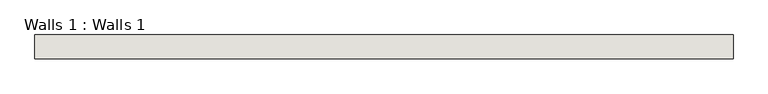
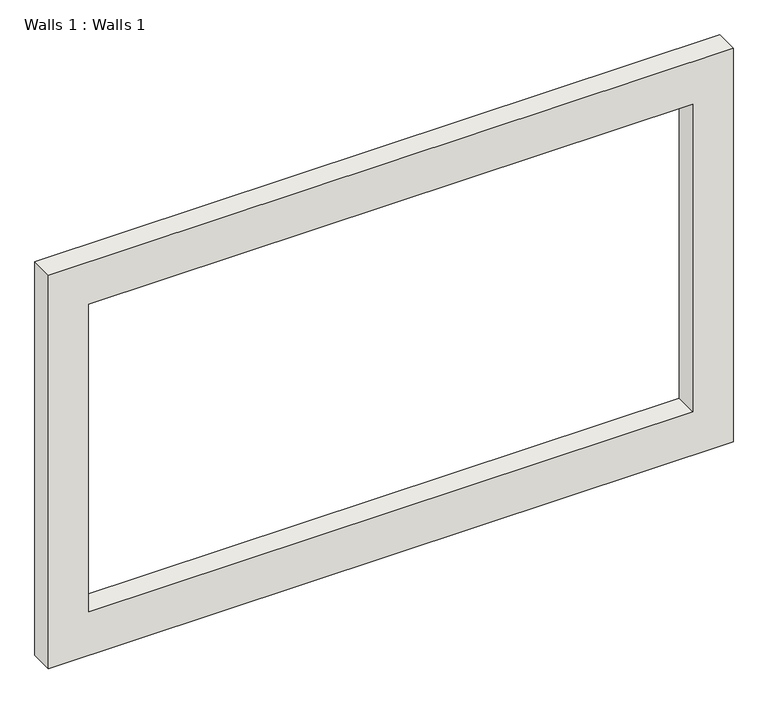
"""IFC4 building model written with IfcOpenShell, lengths in millimetres: wall geometry, Walls 1 : Walls 1."""

from ifc_helpers import new_model, si_unit, frame, origin, place, context, project, spatial, polyline, outline, extrude, source, transform, mapped, element, save


def walls_1_walls_1_d8ce8ff7(model_context):
    return source(origin(), model_context, "Body", "SweptSolid", [
        extrude(outline(polyline([(6661.7693979, 1712.6958607), (6661.7693979, -878.1041393), (5086.9693979, -878.1041393), (5086.9693979, 1712.6958607), (6661.7693979, 1712.6958607)]), holes=[polyline([(6492.024337, 1560.0533085), (5261.1422066, 1560.0533085), (5261.1422066, -725.9466915), (6492.024337, -725.9466915), (6492.024337, 1560.0533085)])]), frame((0.0, -4077.5243623, 0.0), z_axis=(0.0, 1.0, 0.0), x_axis=(0.0, 0.0, 1.0)), (0.0, 0.0, 1.0), 88.2917869),
    ])


if __name__ == "__main__":
    model = new_model("IFC4")
    model_context = context("Model", 3, world=origin())
    ifc_project = project(units=[si_unit("LENGTHUNIT", "METRE", prefix="MILLI")], contexts=[model_context])
    site = spatial("IfcSite", under=ifc_project)
    building = spatial("IfcBuilding", under=site)
    placement = place(None, origin())
    walls_1_walls_1_shape = walls_1_walls_1_d8ce8ff7(model_context)
    element("IfcWall", 1, ObjectType="Walls 1 : Walls 1", at=placement, inside=building, context=model_context, shape_type="MappedRepresentation", body=[
        mapped(walls_1_walls_1_shape, transform((0.0, 0.0, 0.0), x_axis=(1.0, 0.0, 0.0), y_axis=(0.0, 1.0, 0.0), z_axis=(0.0, 0.0, 1.0))),
    ])
    save(model, "model.ifc")

# Revit data of these elements
# Element 1 (IfcWall, "Walls 1 : Walls 1")
#   Materials on its faces: "Default Wall"
# Materials
#   "Default Wall": colour RGB 128 128 128, transparency 0
